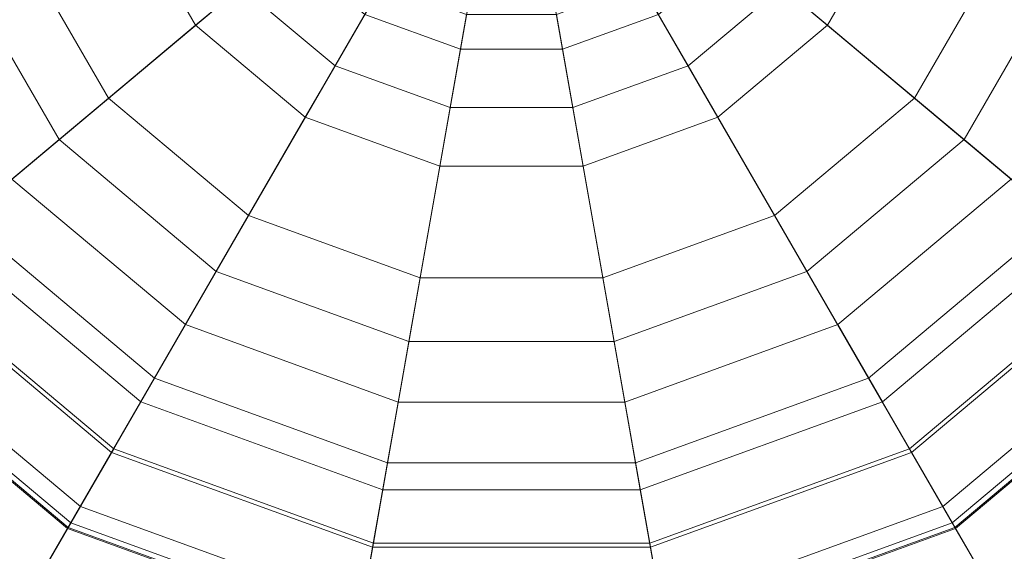
# Model space of a CAD drawing. Units: inches. Extents: x 375 to 1122, y 27 to 1069.
# Tile 140 of 155: x 732.384 to 733.741, y 898.026 to 898.759. Entities that reach past the tile are written whole.
import ezdxf

# ---------------------------------------------------------------- set-up
doc = ezdxf.new("R2010")
doc.units = ezdxf.units.IN
doc.layers.add('A-ANNO-DIMS', color=2, linetype='Continuous', lineweight=18)
doc.layers.add('Furniture', color=30, linetype='Continuous', lineweight=18)
doc.styles.get("Standard").update_dxf_attribs({"font": 'arial.ttf'})
doc.dimstyles.new('ISO-25', dxfattribs={"dimtxt": 12, "dimasz": 2.5, "dimexe": 1.5, "dimexo": 1.5, "dimtad": 1, "dimdec": 1, "dimlunit": 3, "dimtxsty": 'Standard', "dimblk": 'ARCHTICK', "dimcen": 2.5, "dimadec": 0, "dimazin": 0, "dimtfac": 1, "dimtdec": 1, "dimtmove": 0, "dimatfit": 3, "dimfxl": 1.5, "dimfxlon": 1, "dimarcsym": 0})

# ---------------------------------------------------------------- blocks, each defined once
blk = doc.blocks.new('A$C403C54AD')
for points in [[(0.991739, 1.234737, -0.04658), (0.980157, 1.202917, -0.043501), (0.980157, 1.202917, -0.043501), (0.980157, 1.23678, -0.04658)], [(1.001923, 1.228857, -0.04658), (0.980157, 1.202917, -0.043501), (0.980157, 1.202917, -0.043501), (0.991739, 1.234737, -0.04658)], [(0.985019, 1.216274, -0.040074), (0.990622, 1.231669, -0.043349), (0.980157, 1.233514, -0.043349), (0.980157, 1.217132, -0.040074)], [(0.989294, 1.213806, -0.040074), (0.999824, 1.226356, -0.043349), (0.990622, 1.231669, -0.043349), (0.985019, 1.216274, -0.040074)], [(1.009483, 1.219849, -0.04658), (0.980157, 1.202917, -0.043501), (0.980157, 1.202917, -0.043501), (1.001923, 1.228857, -0.04658)], [(1.006655, 1.218216, -0.043349), (1.009483, 1.219849, -0.04658), (1.001923, 1.228857, -0.04658), (0.999824, 1.226356, -0.043349)], [(0.997785, 1.223925, 0.056929), (0.993243, 1.218512, 0.046697), (0.98712, 1.222047, 0.046697), (0.989537, 1.228687, 0.056929)], [(1.00662, 1.218195, 0.116404), (1.009137, 1.219649, 0.10318), (1.001667, 1.228552, 0.10318), (0.999798, 1.226325, 0.116404)], [(1.009137, 1.219649, 0.10318), (1.008553, 1.219312, 0.074938), (1.001233, 1.228035, 0.074938), (1.001667, 1.228552, 0.10318)], [(1.008553, 1.219312, 0.074938), (1.003907, 1.216629, 0.056929), (0.997785, 1.223925, 0.056929), (1.001233, 1.228035, 0.074938)], [(0.991809, 1.216804, 0.048884), (0.995978, 1.221772, 0.058276), (0.988575, 1.226046, 0.058276), (0.986357, 1.219951, 0.048884)], [(0.992467, 1.210025, -0.040074), (1.006655, 1.218216, -0.043349), (0.999824, 1.226356, -0.043349), (0.989294, 1.213806, -0.040074)], [(1.002293, 1.215697, 0.12581), (1.00662, 1.218195, 0.116404), (0.999798, 1.226325, 0.116404), (0.996587, 1.222497, 0.12581)], [(1.006466, 1.218107, 0.102963), (1.004033, 1.216702, 0.115599), (0.997878, 1.224037, 0.115599), (0.999684, 1.226189, 0.102963)], [(1.005896, 1.217778, 0.075423), (1.006466, 1.218107, 0.102963), (0.999684, 1.226189, 0.102963), (0.999261, 1.225685, 0.075423)], [(1.001473, 1.215224, 0.058276), (1.005896, 1.217778, 0.075423), (0.999261, 1.225685, 0.075423), (0.995978, 1.221772, 0.058276)], [(1.004033, 1.216702, 0.115599), (0.999627, 1.214158, 0.12581), (0.994608, 1.220139, 0.12581), (0.997878, 1.224037, 0.115599)], [(1.003907, 1.216629, 0.056929), (0.997787, 1.213096, 0.046697), (0.993243, 1.218512, 0.046697), (0.997785, 1.223925, 0.056929)], [(0.999627, 1.214158, 0.12581), (1.002293, 1.215697, 0.12581), (0.996587, 1.222497, 0.12581), (0.994608, 1.220139, 0.12581)], [(0.993243, 1.218512, 0.046697), (0.986661, 1.210669, 0.03933), (0.983618, 1.212426, 0.03933), (0.98712, 1.222047, 0.046697)], [(0.995856, 1.211981, 0.048884), (1.001473, 1.215224, 0.058276), (0.995978, 1.221772, 0.058276), (0.991809, 1.216804, 0.048884)], [(0.985881, 1.209738, 0.042248), (0.991809, 1.216804, 0.048884), (0.986357, 1.219951, 0.048884), (0.983203, 1.211285, 0.042248)], [(1.013505, 1.208798, -0.04658), (0.980157, 1.202917, -0.043501), (0.980157, 1.202917, -0.043501), (1.009483, 1.219849, -0.04658)], [(1.010249, 1.208223, 0.116404), (1.013112, 1.208728, 0.10318), (1.009137, 1.219649, 0.10318), (1.00662, 1.218195, 0.116404)], [(1.010289, 1.20823, -0.043349), (1.013505, 1.208798, -0.04658), (1.009483, 1.219849, -0.04658), (1.006655, 1.218216, -0.043349)], [(1.012448, 1.208611, 0.074938), (1.007164, 1.20768, 0.056929), (1.003907, 1.216629, 0.056929), (1.008553, 1.219312, 0.074938)], [(0.997787, 1.213096, 0.046697), (0.98892, 1.207977, 0.03933), (0.986661, 1.210669, 0.03933), (0.993243, 1.218512, 0.046697)], [(0.994156, 1.205386, -0.040074), (1.010289, 1.20823, -0.043349), (1.006655, 1.218216, -0.043349), (0.992467, 1.210025, -0.040074)], [(1.005329, 1.207356, 0.12581), (1.010249, 1.208223, 0.116404), (1.00662, 1.218195, 0.116404), (1.002293, 1.215697, 0.12581)], [(1.010075, 1.208193, 0.102963), (1.007308, 1.207705, 0.115599), (1.004033, 1.216702, 0.115599), (1.006466, 1.218107, 0.102963)], [(1.009426, 1.208078, 0.075423), (1.010075, 1.208193, 0.102963), (1.006466, 1.218107, 0.102963), (1.005896, 1.217778, 0.075423)], [(1.004396, 1.207191, 0.058276), (1.009426, 1.208078, 0.075423), (1.005896, 1.217778, 0.075423), (1.001473, 1.215224, 0.058276)], [(0.987868, 1.207369, 0.042248), (0.995856, 1.211981, 0.048884), (0.991809, 1.216804, 0.048884), (0.985881, 1.209738, 0.042248)], [(1.007164, 1.20768, 0.056929), (1.000206, 1.206452, 0.046697), (0.997787, 1.213096, 0.046697), (1.003907, 1.216629, 0.056929)], [(1.007308, 1.207705, 0.115599), (1.002297, 1.206821, 0.12581), (0.999627, 1.214158, 0.12581), (1.004033, 1.216702, 0.115599)], [(0.987978, 1.212238, -0.037209), (0.989294, 1.213806, -0.040074), (0.985019, 1.216274, -0.040074), (0.984318, 1.21435, -0.037209)], [(1.002297, 1.206821, 0.12581), (1.005329, 1.207356, 0.12581), (1.002293, 1.215697, 0.12581), (0.999627, 1.214158, 0.12581)], [(0.998009, 1.206065, 0.048884), (1.004396, 1.207191, 0.058276), (1.001473, 1.215224, 0.058276), (0.995856, 1.211981, 0.048884)], [(0.990694, 1.209001, -0.037209), (0.992467, 1.210025, -0.040074), (0.989294, 1.213806, -0.040074), (0.987978, 1.212238, -0.037209)], [(1.000206, 1.206452, 0.046697), (0.990122, 1.204675, 0.03933), (0.98892, 1.207977, 0.03933), (0.997787, 1.213096, 0.046697)], [(0.987147, 1.206953, -0.035163), (0.990694, 1.209001, -0.037209), (0.987978, 1.212238, -0.037209), (0.985345, 1.2091, -0.035163)], [(0.988926, 1.204464, 0.042248), (0.998009, 1.206065, 0.048884), (0.995856, 1.211981, 0.048884), (0.987868, 1.207369, 0.042248)], [(0.992139, 1.20503, -0.037209), (0.994156, 1.205386, -0.040074), (0.992467, 1.210025, -0.040074), (0.990694, 1.209001, -0.037209)], [(1.013505, 1.197037, -0.04658), (0.980157, 1.202917, -0.043501), (0.980157, 1.202917, -0.043501), (1.013505, 1.208798, -0.04658)], [(0.988106, 1.204319, -0.035163), (0.992139, 1.20503, -0.037209), (0.990694, 1.209001, -0.037209), (0.987147, 1.206953, -0.035163)], [(1.012448, 1.197224, 0.074938), (1.007164, 1.198155, 0.056929), (1.007164, 1.20768, 0.056929), (1.012448, 1.208611, 0.074938)], [(0.994156, 1.200449, -0.040074), (1.010289, 1.197604, -0.043349), (1.010289, 1.20823, -0.043349), (0.994156, 1.205386, -0.040074)], [(1.004396, 1.198643, 0.058276), (1.009426, 1.197756, 0.075423), (1.009426, 1.208078, 0.075423), (1.004396, 1.207191, 0.058276)], [(1.005329, 1.198479, 0.12581), (1.010249, 1.197611, 0.116404), (1.010249, 1.208223, 0.116404), (1.005329, 1.207356, 0.12581)], [(1.010075, 1.197642, 0.102963), (1.007308, 1.19813, 0.115599), (1.007308, 1.207705, 0.115599), (1.010075, 1.208193, 0.102963)], [(0.990122, 1.204675, 0.03933), (0.985282, 1.203821, 0.038511), (0.984664, 1.205519, 0.038511), (0.98892, 1.207977, 0.03933)], [(1.007308, 1.19813, 0.115599), (1.002297, 1.199014, 0.12581), (1.002297, 1.206821, 0.12581), (1.007308, 1.207705, 0.115599)], [(1.007164, 1.198155, 0.056929), (1.000206, 1.199382, 0.046697), (1.000206, 1.206452, 0.046697), (1.007164, 1.20768, 0.056929)], [(0.998009, 1.19977, 0.048884), (1.004396, 1.198643, 0.058276), (1.004396, 1.207191, 0.058276), (0.998009, 1.206065, 0.048884)], [(1.002297, 1.199014, 0.12581), (1.005329, 1.198479, 0.12581), (1.005329, 1.207356, 0.12581), (1.002297, 1.206821, 0.12581)], [(1.000206, 1.199382, 0.046697), (0.990122, 1.20116, 0.03933), (0.990122, 1.204675, 0.03933), (1.000206, 1.206452, 0.046697)], [(0.988926, 1.201371, 0.042248), (0.998009, 1.19977, 0.048884), (0.998009, 1.206065, 0.048884), (0.988926, 1.204464, 0.042248)], [(0.992139, 1.200805, -0.037209), (0.994156, 1.200449, -0.040074), (0.994156, 1.205386, -0.040074), (0.992139, 1.20503, -0.037209)], [(0.988106, 1.201516, -0.035163), (0.992139, 1.200805, -0.037209), (0.992139, 1.20503, -0.037209), (0.988106, 1.204319, -0.035163)], [(0.990122, 1.20116, 0.03933), (0.985282, 1.202014, 0.038511), (0.985282, 1.203821, 0.038511), (0.990122, 1.204675, 0.03933)], [(1.009483, 1.185986, -0.04658), (0.980157, 1.202917, -0.043501), (0.980157, 1.202917, -0.043501), (1.013505, 1.197037, -0.04658)], [(1.001923, 1.176977, -0.04658), (0.980157, 1.202917, -0.043501), (0.980157, 1.202917, -0.043501), (1.009483, 1.185986, -0.04658)], [(0.991739, 1.171097, -0.04658), (0.980157, 1.202917, -0.043501), (0.980157, 1.202917, -0.043501), (1.001923, 1.176977, -0.04658)], [(0.980157, 1.169055, -0.04658), (0.980157, 1.202917, -0.043501), (0.980157, 1.202917, -0.043501), (0.991739, 1.171097, -0.04658)], [(0.98892, 1.197858, 0.03933), (0.984664, 1.200315, 0.038511), (0.985282, 1.202014, 0.038511), (0.990122, 1.20116, 0.03933)], [(0.987147, 1.198882, -0.035163), (0.990694, 1.196834, -0.037209), (0.992139, 1.200805, -0.037209), (0.988106, 1.201516, -0.035163)], [(0.987868, 1.198465, 0.042248), (0.995856, 1.193854, 0.048884), (0.998009, 1.19977, 0.048884), (0.988926, 1.201371, 0.042248)], [(0.997787, 1.192739, 0.046697), (0.98892, 1.197858, 0.03933), (0.990122, 1.20116, 0.03933), (1.000206, 1.199382, 0.046697)], [(0.990694, 1.196834, -0.037209), (0.992467, 1.19581, -0.040074), (0.994156, 1.200449, -0.040074), (0.992139, 1.200805, -0.037209)], [(0.992467, 1.19581, -0.040074), (1.006655, 1.187619, -0.043349), (1.010289, 1.197604, -0.043349), (0.994156, 1.200449, -0.040074)], [(0.995856, 1.193854, 0.048884), (1.001473, 1.190611, 0.058276), (1.004396, 1.198643, 0.058276), (0.998009, 1.19977, 0.048884)], [(1.003907, 1.189206, 0.056929), (0.997787, 1.192739, 0.046697), (1.000206, 1.199382, 0.046697), (1.007164, 1.198155, 0.056929)], [(0.985345, 1.196735, -0.035163), (0.987978, 1.193597, -0.037209), (0.990694, 1.196834, -0.037209), (0.987147, 1.198882, -0.035163)], [(0.999627, 1.191677, 0.12581), (1.002293, 1.190138, 0.12581), (1.005329, 1.198479, 0.12581), (1.002297, 1.199014, 0.12581)], [(1.004033, 1.189133, 0.115599), (0.999627, 1.191677, 0.12581), (1.002297, 1.199014, 0.12581), (1.007308, 1.19813, 0.115599)], [(1.001473, 1.190611, 0.058276), (1.005896, 1.188057, 0.075423), (1.009426, 1.197756, 0.075423), (1.004396, 1.198643, 0.058276)], [(0.985881, 1.196096, 0.042248), (0.991809, 1.189031, 0.048884), (0.995856, 1.193854, 0.048884), (0.987868, 1.198465, 0.042248)], [(1.002293, 1.190138, 0.12581), (1.00662, 1.187639, 0.116404), (1.010249, 1.197611, 0.116404), (1.005329, 1.198479, 0.12581)], [(0.993243, 1.187323, 0.046697), (0.986661, 1.195166, 0.03933), (0.98892, 1.197858, 0.03933), (0.997787, 1.192739, 0.046697)], [(1.008553, 1.186523, 0.074938), (1.003907, 1.189206, 0.056929), (1.007164, 1.198155, 0.056929), (1.012448, 1.197224, 0.074938)], [(1.006466, 1.187728, 0.102963), (1.004033, 1.189133, 0.115599), (1.007308, 1.19813, 0.115599), (1.010075, 1.197642, 0.102963)], [(1.005896, 1.188057, 0.075423), (1.006466, 1.187728, 0.102963), (1.010075, 1.197642, 0.102963), (1.009426, 1.197756, 0.075423)], [(1.00662, 1.187639, 0.116404), (1.009137, 1.186186, 0.10318), (1.013112, 1.197107, 0.10318), (1.010249, 1.197611, 0.116404)], [(1.006655, 1.187619, -0.043349), (1.009483, 1.185986, -0.04658), (1.013505, 1.197037, -0.04658), (1.010289, 1.197604, -0.043349)], [(0.987978, 1.193597, -0.037209), (0.989294, 1.192029, -0.040074), (0.992467, 1.19581, -0.040074), (0.990694, 1.196834, -0.037209)], [(0.983203, 1.19455, 0.042248), (0.986357, 1.185883, 0.048884), (0.991809, 1.189031, 0.048884), (0.985881, 1.196096, 0.042248)], [(0.989294, 1.192029, -0.040074), (0.999824, 1.179479, -0.043349), (1.006655, 1.187619, -0.043349), (0.992467, 1.19581, -0.040074)], [(0.98712, 1.183788, 0.046697), (0.983618, 1.193409, 0.03933), (0.986661, 1.195166, 0.03933), (0.993243, 1.187323, 0.046697)], [(0.991809, 1.189031, 0.048884), (0.995978, 1.184063, 0.058276), (1.001473, 1.190611, 0.058276), (0.995856, 1.193854, 0.048884)], [(0.984318, 1.191485, -0.037209), (0.985019, 1.18956, -0.040074), (0.989294, 1.192029, -0.040074), (0.987978, 1.193597, -0.037209)], [(0.997785, 1.18191, 0.056929), (0.993243, 1.187323, 0.046697), (0.997787, 1.192739, 0.046697), (1.003907, 1.189206, 0.056929)], [(0.985019, 1.18956, -0.040074), (0.990622, 1.174166, -0.043349), (0.999824, 1.179479, -0.043349), (0.989294, 1.192029, -0.040074)], [(0.994608, 1.185696, 0.12581), (0.996587, 1.183338, 0.12581), (1.002293, 1.190138, 0.12581), (0.999627, 1.191677, 0.12581)], [(0.997878, 1.181798, 0.115599), (0.994608, 1.185696, 0.12581), (0.999627, 1.191677, 0.12581), (1.004033, 1.189133, 0.115599)], [(0.995978, 1.184063, 0.058276), (0.999261, 1.18015, 0.075423), (1.005896, 1.188057, 0.075423), (1.001473, 1.190611, 0.058276)], [(0.996587, 1.183338, 0.12581), (0.999798, 1.17951, 0.116404), (1.00662, 1.187639, 0.116404), (1.002293, 1.190138, 0.12581)], [(0.980157, 1.188703, -0.040074), (0.980157, 1.172321, -0.043349), (0.990622, 1.174166, -0.043349), (0.985019, 1.18956, -0.040074)], [(1.001233, 1.1778, 0.074938), (0.997785, 1.18191, 0.056929), (1.003907, 1.189206, 0.056929), (1.008553, 1.186523, 0.074938)], [(0.999684, 1.179646, 0.102963), (0.997878, 1.181798, 0.115599), (1.004033, 1.189133, 0.115599), (1.006466, 1.187728, 0.102963)], [(0.986357, 1.185883, 0.048884), (0.988575, 1.179789, 0.058276), (0.995978, 1.184063, 0.058276), (0.991809, 1.189031, 0.048884)], [(0.999261, 1.18015, 0.075423), (0.999684, 1.179646, 0.102963), (1.006466, 1.187728, 0.102963), (1.005896, 1.188057, 0.075423)], [(0.999798, 1.17951, 0.116404), (1.001667, 1.177283, 0.10318), (1.009137, 1.186186, 0.10318), (1.00662, 1.187639, 0.116404)], [(0.999824, 1.179479, -0.043349), (1.001923, 1.176977, -0.04658), (1.009483, 1.185986, -0.04658), (1.006655, 1.187619, -0.043349)], [(0.989537, 1.177147, 0.056929), (0.98712, 1.183788, 0.046697), (0.993243, 1.187323, 0.046697), (0.997785, 1.18191, 0.056929)], [(1.001667, 1.177283, 0.10318), (1.001233, 1.1778, 0.074938), (1.008553, 1.186523, 0.074938), (1.009137, 1.186186, 0.10318)]]:
    blk.add_3dface(points)
blk = doc.blocks.new('_ArchTick')
at = {"color": 0, "linetype": 'ByBlock', "const_width": 0.15}
blk.add_lwpolyline([(-0.5, -0.5), (0.5, 0.5)], dxfattribs=at)
blk = doc.blocks.new('*D88')
at = {"layer": 'A-ANNO-DIMS', "color": 0, "lineweight": -2, "transparency": 16777216}
for p, q in [((731.0073, 1052.5277), (731.0073, 1055.5277)), ((854.0073, 1052.5277), (854.0073, 1055.5277)), ((731.0073, 1054.0277), (854.0073, 1054.0277))]:
    blk.add_line(p, q, dxfattribs=at)
at = {"layer": 'Defpoints', "color": 0, "transparency": 16777216}
for p in [(854.0073, 1054.0277), (731.0073, 502.5277), (854.0073, 502.5277)]:
    blk.add_point(p, dxfattribs=at)
at = {"layer": 'A-ANNO-DIMS', "color": 0, "lineweight": -2, "transparency": 16777216, "xscale": 2.5, "yscale": 2.5, "zscale": 2.5, "rotation": 180}
blk.add_blockref('_ArchTick', (731.0073, 1054.0277), dxfattribs=at)
at = {"layer": 'A-ANNO-DIMS', "color": 0, "lineweight": -2, "transparency": 16777216, "xscale": 2.5, "yscale": 2.5, "zscale": 2.5}
blk.add_blockref('_ArchTick', (854.0073, 1054.0277), dxfattribs=at)
at = {"layer": 'A-ANNO-DIMS', "color": 0, "transparency": 16777216, "insert": (792.5073, 1060.7837), "char_height": 12, "attachment_point": 5}
blk.add_mtext('10\'-3"', dxfattribs=at)
blk = doc.blocks.new('*D91')
at = {"layer": 'A-ANNO-DIMS', "color": 0, "lineweight": -2, "transparency": 16777216}
for p, q in [((728.0073, 1052.5277), (728.0073, 1055.5277)), ((788.0073, 1052.5277), (788.0073, 1055.5277)), ((728.0073, 1054.0277), (788.0073, 1054.0277))]:
    blk.add_line(p, q, dxfattribs=at)
at = {"layer": 'Defpoints', "color": 0, "transparency": 16777216}
for p in [(788.0073, 1054.0277), (728.0073, 774.0277), (788.0073, 774.0277)]:
    blk.add_point(p, dxfattribs=at)
at = {"layer": 'A-ANNO-DIMS', "color": 0, "lineweight": -2, "transparency": 16777216, "xscale": 2.5, "yscale": 2.5, "zscale": 2.5, "rotation": 180}
blk.add_blockref('_ArchTick', (728.0073, 1054.0277), dxfattribs=at)
at = {"layer": 'A-ANNO-DIMS', "color": 0, "lineweight": -2, "transparency": 16777216, "xscale": 2.5, "yscale": 2.5, "zscale": 2.5}
blk.add_blockref('_ArchTick', (788.0073, 1054.0277), dxfattribs=at)
at = {"layer": 'A-ANNO-DIMS', "color": 0, "transparency": 16777216, "insert": (758.0073, 1060.7796), "char_height": 12, "attachment_point": 5}
blk.add_mtext('5\'-0"', dxfattribs=at)

msp = doc.modelspace()

# ---------------------------------------------------------------- block references
at = {"layer": 'Furniture', "xscale": 39.9918517141215, "yscale": 39.9918517141215, "zscale": 39.9918517141215, "rotation": 270}
msp.add_blockref('A$C403C54AD', (684.9549, 938.3156, 0.024), dxfattribs=at)

# ---------------------------------------------------------------- dimensions: what is measured, and where the dimension line sits
at = {"layer": 'A-ANNO-DIMS'}
for base, p1, p2, picture, middle in [((854.0073, 1054.0277), (731.0073, 502.5277), (854.0073, 502.5277), '*D88', (792.5073, 1060.7837)), ((788.0073, 1054.0277), (728.0073, 774.0277), (788.0073, 774.0277), '*D91', (758.0073, 1060.7796))]:
    dim = msp.add_linear_dim(base=base, p1=p1, p2=p2, dimstyle='ISO-25', override={"dimdec": 1, "dimlfac": 1, "dimrnd": 0, "dimzin": 1, "dimdsep": 46, "dimlunit": 4, "dimfrac": 2}, dxfattribs=at)
    dim.commit()
    dim.dimension.update_dxf_attribs({"geometry": picture, "text_midpoint": middle})

doc.saveas('drawing.dxf')
